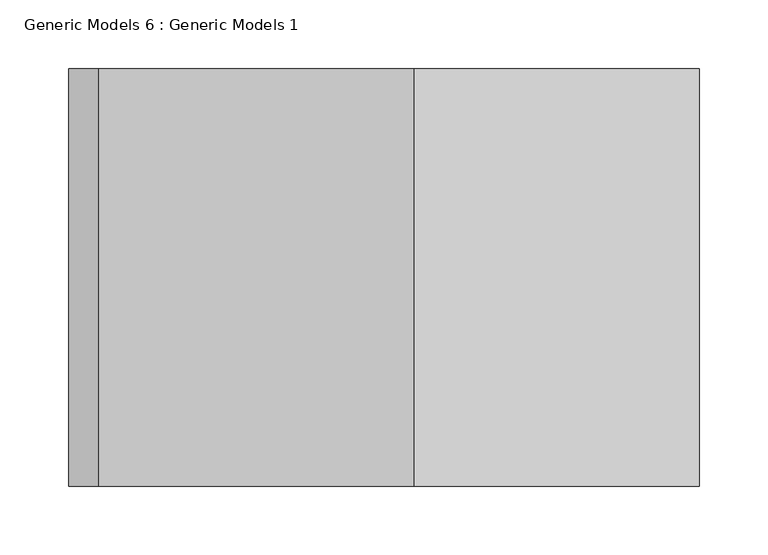
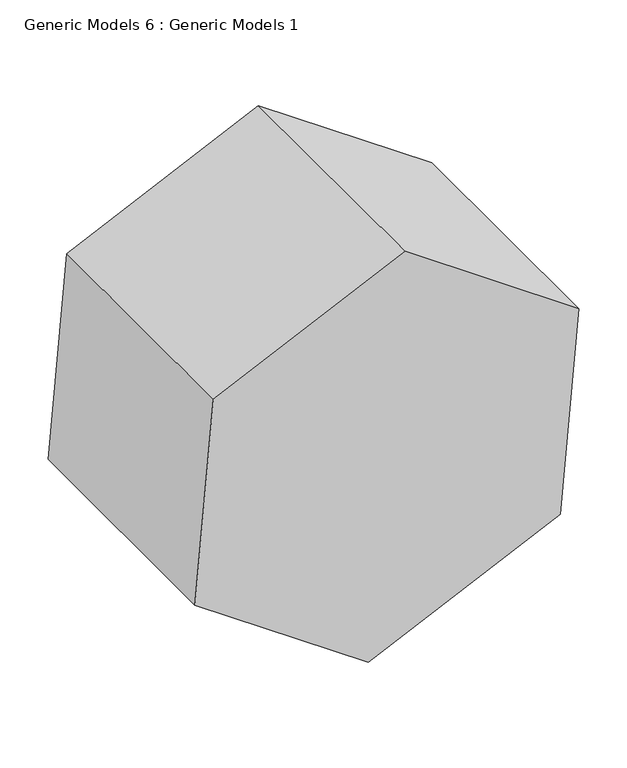
"""IFC4 building model written with IfcOpenShell, lengths in millimetres: proxy geometry, Generic Models 6 : Generic Models 1."""

from ifc_helpers import new_model, si_unit, frame, origin, place, context, project, spatial, polyline, outline, extrude, source, transform, mapped, element, save


def generic_models_6_generic_models_1_f976f914(model_context):
    return source(origin(), model_context, "Body", "SweptSolid", [
        extrude(outline(polyline([(833.1013393, -3610.3079055), (978.7897542, -3818.3725247), (871.4447157, -4048.5747026), (618.4112624, -4070.7122613), (472.7228475, -3862.647642), (580.067886, -3632.4454641), (833.1013393, -3610.3079055)])), frame((0.0, -10720.3372434, 0.0), z_axis=(0.0, 1.0, 0.0), x_axis=(0.0, 0.0, 1.0)), (0.0, 0.0, 1.0), 304.8),
    ])


if __name__ == "__main__":
    model = new_model("IFC4")
    model_context = context("Model", 3, world=origin())
    ifc_project = project(units=[si_unit("LENGTHUNIT", "METRE", prefix="MILLI")], contexts=[model_context])
    site = spatial("IfcSite", under=ifc_project)
    building = spatial("IfcBuilding", under=site)
    placement = place(None, origin())
    generic_models_6_generic_models_1_shape = generic_models_6_generic_models_1_f976f914(model_context)
    element("IfcBuildingElementProxy", 1, Name="Generic Models 6 : Generic Models 1", ObjectType="Generic Models 6 : Generic Models 1", at=placement, inside=building, context=model_context, shape_type="MappedRepresentation", body=[
        mapped(generic_models_6_generic_models_1_shape, transform((0.0, 0.0, 0.0), x_axis=(1.0, 0.0, 0.0), y_axis=(0.0, 1.0, 0.0), z_axis=(0.0, 0.0, 1.0))),
    ])
    save(model, "model.ifc")

# Revit data of these elements
# Element 1 (IfcBuildingElementProxy, "Generic Models 6 : Generic Models 1")
#   Materials on its faces: "Carpet (1)"
# Materials
#   "Carpet (1)": class "Carpet", colour RGB 124 80 67, transparency 0, Description = "Interior finish", Cost = 0
